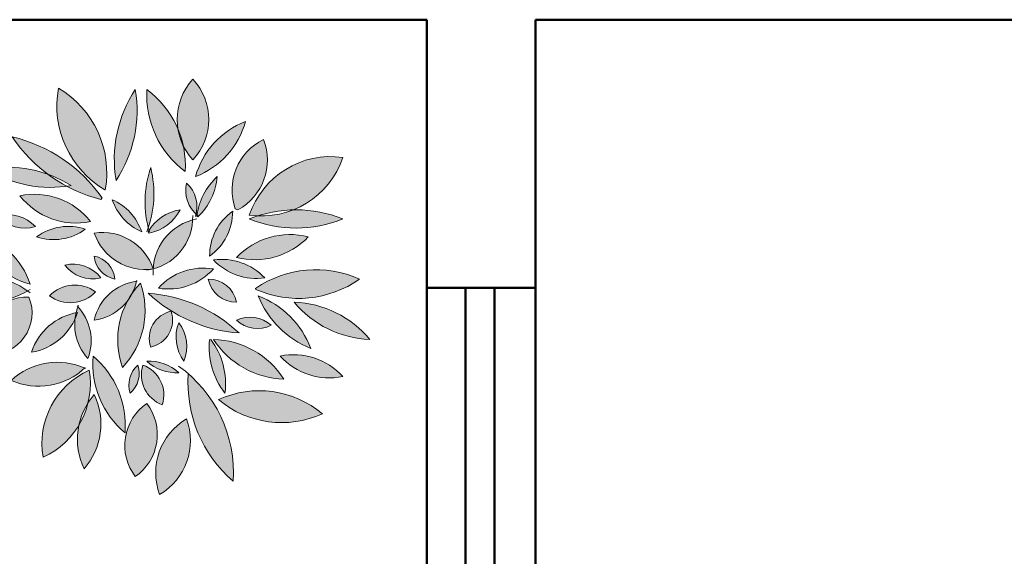
# Model space of a CAD drawing. Units: inches. Extents: x 64 to 1167, y 117 to 939.
# Tile 25 of 56: x 358 to 394, y 837 to 857. Entities that reach past the tile are written whole.
import ezdxf

# ---------------------------------------------------------------- set-up
doc = ezdxf.new("R2010")
doc.units = ezdxf.units.IN
doc.header["$MEASUREMENT"] = 0
doc.layers.add('A-FURN', color=8, linetype='Continuous', lineweight=18)
doc.layers.add('A-WALL', color=7, linetype='Continuous', lineweight=50)

# ---------------------------------------------------------------- blocks, each defined once
blk = doc.blocks.new('A$C172C5132')
at = {"linetype": 'ByBlock'}
h = blk.add_hatch(color=256, dxfattribs=at)
h.set_gradient(color1=(15, 138, 17), color2=(46, 92, 10), tint=1, name='HEMISPHERICAL')
h.paths.add_polyline_path([(0.0848516368565885, 0.0409433570912889, 0.2362815525011606), (0.1000330567823523, 0.0044683605559084, 0.2362815525011239)])
h.paths.add_polyline_path([(0.0951251289552244, 0.0321643424477881, 0.2906279390332829), (0.1303084046611637, 0.0273831593592676, 0.290627939033283)])
h.paths.add_polyline_path([(0.0751445134197123, 6.9582163e-09, 0.3640818940120694), (0.0842661026749416, 0.0256445447606496, 0.3640818940120696)])
h.paths.add_polyline_path([(0.0708009012055837, 0.0308603718690661, 0.4289359753156656), (0.0668916470544005, 0.0060851551611861, 0.4289359753156655)])
h.paths.add_polyline_path([(0.0525577128238133, 0.046942555388035, 0.2430552989308659), (0.0634167555244858, 0.0208633514542425, 0.2430552989308659)])
h.paths.add_polyline_path([(0.0508922599916389, 0.0310927787270394, -0.075691505353723), (0.0477797489950209, 0.0234712737617285, 0.1646663790635834), (0.0495171986775909, 0.0086930668678311, 0.2986360287318925), (0.0529920876610994, 0.0339029598950939, 0.0378503895202349)])
h.paths.add_polyline_path([(0.0356176258998936, 0.0126049410038033, 0.1525669483622997), (0.0477797489950209, 0.0234712737618002, -0.0894079227445343), (0.0508922599916389, 0.0310927787270394, 0.1023004185508453), (0.0512546390377685, 0.0421613668636365, 0.3412881037578929)])
h.paths.add_polyline_path([(0.0247586152468425, 0.0386841445389578, 0.2992020634273156), (0.0497584931614385, 0.0428499944584606, 0.2992020634272661)])
h.paths.add_polyline_path([(0.047451336783066, 0.0636633223899126, 0.031181829370212), (0.0468224604404838, 0.0616275993652971, -0.0067074306643478), (0.047345392022932, 0.0617207568240691), (0.0473453770955458, 0.0617207543709398), (0.0473453802906652, 0.0617207643046988, -0.0313798428369172), (0.0464385188093715, 0.0594096693237134, 0.214704016687058), (0.0508202830851731, 0.0460732317601093, 0.2827951388784949)])
h.paths.add_polyline_path([(0.0643270393991799, 0.0657681421224303, 0.2116588201392034), (0.0625480317599852, 0.0430306771320518, 0.2810507069368319), (0.0686290949419001, 0.0717177787730742, 0.0387724880797508), (0.0658907288251662, 0.0683269518706705, -0.0447168196076769)])
h.paths.add_polyline_path([(0.0529920908817849, 0.0591128495135777, 0.2037329938010539), (0.0643270393991799, 0.0657681421224303, -0.0266555720820853), (0.0658907288251304, 0.0683269518706347, 0.0628291983769196), (0.0672680139649763, 0.0723002515858513, 0.3185820290807026)])
h.paths.add_polyline_path([(0.0694978092295733, 0.0438999815920186, 0.4032574184254003), (0.0760132376538916, 0.0304257186990447, 0.4032574184254003)])
h.paths.add_polyline_path([(0.0651542049250408, 0.0343376032784868, 0.3026067215504981), (0.0677603739667911, 0.0438999851589565, 0.3026067215504981)])
h.paths.add_polyline_path([(0.0708009089365751, 0.0452039393599706, 0.2041900440368323), (0.0816599225525022, 0.0412920661897099, 0.2041900440368324)])
h.paths.add_polyline_path([(0.081659931129825, 0.0582435357128855, 0.2621375963259251), (0.0833973804279365, 0.0452039328038387, 0.2621375963259252)])
h.paths.add_polyline_path([(0.0721039783237091, 0.0499851199959349, 0.4463603731284183), (0.0790537760999147, 0.0621554185296266, 0.4463603731284183)])
h.paths.add_polyline_path([(0.0933876910232543, 0.0525930422323801, 0.2470851436575526), (0.117277559364148, 0.0391187980764294, 0.2470851436575526)])
h.paths.add_polyline_path([(0.0712352546233386, 0.068240566365182, 0.1714668564556485), (0.1020749306824684, 0.054766306652217, 0.1714668564556485)])
h.paths.add_polyline_path([(0.0747101479397659, 0.0699791674706583, 0.2592783200943487), (0.0933876928733241, 0.0764989740396572, 0.2592783200943487)])
h.paths.add_polyline_path([(0.0916502366687461, 0.0730217515827079, 0.3656390256905797), (0.101206201234342, 0.0651979848924216, 0.3656390256905797)])
h.paths.add_polyline_path([(0.0933876912086265, 0.0795415399056317, 0.2434153457947699), (0.1107621376206411, 0.0734563950534696, 0.2434153457947698)])
h.paths.add_polyline_path([(0.1012061854802825, 0.0591128377539187, 0.3074508191165638), (0.1129339572098902, 0.0573742297376074, 0.3074508191165636)])
h.paths.add_polyline_path([(0.1085903436375709, 0.0673712529429685, 0.2096325949128592), (0.1263991528693673, 0.0495504795221731, 0.2096325949128592)])
h.paths.add_polyline_path([(0.1207524492141115, 0.065197986908134, 0.2131103218534129), (0.1463797799587205, 0.0525930392730849, 0.2131103218534128)])
h.paths.add_polyline_path([(0.1159744952746058, 0.0469425441179992, 0.2657190469918038), (0.1372581767641242, 0.039988102251266, 0.2657190469918037)])
h.paths.add_polyline_path([(0.1012062017913538, 0.0804108456417557, 0.2715342573869963), (0.1255304209675389, 0.0873652998785119, 0.2715342573869963)])
h.paths.add_polyline_path([(0.1203979563089573, 0.0965262847971841, -0.1054095226912168), (0.1084157654269272, 0.0944920995295244, 0.018051737402885), (0.1055497991297656, 0.0934504485621891, 0.1947634324622436), (0.1372581839236379, 0.0934504485621891, 0.1024884098922396)])
h.paths.add_polyline_path([(0.1055498097535589, 0.0947544097676372, 0.0247013481528025), (0.1084157654269988, 0.0944920995295244, -0.0722993566674296), (0.1203979563089573, 0.0965262847971841, 0.2204439691458661), (0.1372581853767884, 0.1143137971598573, 0.3612839562176665)])
h.paths.add_polyline_path([(0.0920846062711383, 0.0808455117020383, 0.2441882660981068), (0.0999031055369228, 0.0960583567237383, 0.2441882660981067)])
h.paths.add_polyline_path([(0.0873066344977665, 0.1077940073224099, 0.2360393724983017), (0.104246714262817, 0.1264840796844728, 0.2360393724983016)])
h.paths.add_polyline_path([(0.0842661033232609, 0.1056207182491079, 0.2718871002718489), (0.0875115893454784, 0.0950658132315734, 0.2718871002715955)])
h.paths.add_polyline_path([(0.0729522379931478, 0.076559000959958, -0.0011928136807371), (0.072980246539008, 0.0764766754647066, 0.3253441804237751), (0.0863528333196324, 0.0931339331977748, 0.3244683045754948)])
h.paths.add_polyline_path([(0.0712894635586684, 0.0904598878984896, 0.1439511720342415), (0.0721039819483319, 0.1108365706518253, 0.1439511720343805)])
h.paths.add_polyline_path([(0.0590731413665092, 0.0999702409597207, 0.2079760795555611), (0.0690634560800835, 0.0891039085706064, 0.207976079555561)])
h.paths.add_polyline_path([(0.0603762293124555, 0.1064900535994177, 0.1901074032574417), (0.0668916420391818, 0.137350397132487, 0.1901074032574415)])
h.paths.add_polyline_path([(0.0708008986345782, 0.1373504136971785, 0.2529037224987196), (0.0838317360148722, 0.1095326193878703, 0.0679209033287059), (0.083148370263475, 0.1182431328493921, -0.0747956075290694), (0.0813338508249389, 0.1239670055877479, 0.1341585858806744)])
h.paths.add_polyline_path([(0.0813338508249389, 0.1239670055877479, -0.0465642878043537), (0.083148370263475, 0.1182431328493921, 0.0724450463034802), (0.086437905090639, 0.1134444986822172, 0.3910737637767219), (0.086437905090639, 0.140827633644925, 0.2297305268739758)])
h = blk.add_hatch(color=256, dxfattribs=at)
h.set_gradient(color1=(12, 110, 14), color2=(39, 78, 9), tint=1, name='HEMISPHERICAL')
h.paths.add_polyline_path([(0.0277991349999923, 0.1012741996741918, 0.2872652564561664), (0.0516889943617385, 0.0925811437956438, 0.2872652564561664)])
h.paths.add_polyline_path([(0.0334458088073508, 0.0873652986886136, 0.2454535408657207), (0.0499515759045565, 0.089973222633763, 0.2454535408657209)])
h.paths.add_polyline_path([(0.0529920764399042, 0.0886692609657258, 0.3628842943462125), (0.0729490150136937, 0.0764954078429701, -0.0008769890010568), (0.0729522379931478, 0.076559000959958, 0.362271709300998)])
h.paths.add_polyline_path([(0.052992082253688, 0.0808454969822246, 0.3332704001676869), (0.0599418568393184, 0.0730217437701484, 0.3332704001676869)])
h.paths.add_polyline_path([(0.0430017763078933, 0.0778029274210876, 0.3029447989434044), (0.055163891633107, 0.0734563959517209, 0.3029447989434045)])
h.paths.add_polyline_path([(0.0377894338124123, 0.0673712519411278, 0.378762981535274), (0.0534264495230472, 0.0686752079740218, 0.378762981535274)])
h.paths.add_polyline_path([(0.0317083892186356, 0.0482465196716572, 0.2476978196244638), (0.0464385188093715, 0.059409669323785, -0.03294569524484), (0.046822460440448, 0.0616275993652971, 0.2740394890495783)])
h.paths.add_polyline_path([(0.0169400999274739, 0.0473772010126878, 0.5498076116501301), (0.0308396477386464, 0.0669366019959097, 0.5498076116501304)])
h.paths.add_polyline_path([(5.8794536e-09, 0.0704138252261443, 0.2977812259051555), (0.030406089434854, 0.069011140085252, 0.2977812259051677)])
h.paths.add_polyline_path([(0.0130308377588801, 0.0886692600222146, 0.2481107794618412), (0.0312740176044698, 0.0712831333595387, 0.2481107794618409)])
h.paths.add_polyline_path([(0.0204149782987906, 0.0943197520353183, 0.2904151352643436), (0.0330114769075243, 0.09084252142568, 0.2904151352643436)])
h.paths.add_polyline_path([(0.0165057375983538, 0.1104019119840517, 0.1754058278069592), (0.0436644963260339, 0.1045192247680393, -0.0373225713202712), (0.0372078839723324, 0.1086182328550855, 0.1293741954878769)])
h.paths.add_polyline_path([(0.0251929565725431, 0.1212682457447485, 0.0856466426118782), (0.0372078839723682, 0.1086182328550855, -0.0543838481538954), (0.04517356720194, 0.1047514234187564), (0.0451735772956124, 0.1047514251656665, -0.009350805838724), (0.0436644963260339, 0.1045192247680393, 0.0605073730854804), (0.0551972396525293, 0.1000437593582652), (0.0556053915159454, 0.1006328511779318, 0.1852537253176007)])
h.paths.add_polyline_path([(0.0408299697457594, 0.137785076184794, 0.3132662906545535), (0.0565859837452511, 0.103262326620679), (0.0567280634683676, 0.1033275296575847, 0.313266248548697)])
h.paths.add_polyline_path([(0.0712352633028543, 0.0891039098711838), (0.0715593597632914, 0.0886487531724155, 0.2302319040247018), (0.0820942930736631, 0.0964930128417399, 0.2302320083900739)])
h.paths.add_polyline_path([(0.0877409962472449, 0.094319752764776), (0.0881219586038091, 0.0941299738834785, 0.1793447999456611), (0.0946907683226341, 0.1077939919612951, 0.179344717845649)])
h.paths.add_polyline_path([(0.1007774209509037, 0.0968245554685736), (0.1016405548364666, 0.0964930185287673, 0.3782823007975571), (0.110327781776827, 0.120398949988467, 0.3782823000244757)])
h = blk.add_hatch(color=256, dxfattribs=at)
h.set_gradient(color1=(12, 110, 14), color2=(39, 78, 9), tint=1, name='HEMISPHERICAL')
h.paths.add_polyline_path([(0.1076878936631927, 0.0699044517198683), (0.1077216139834834, 0.0695445217982392, 0.2622438465353351), (0.1429048742833344, 0.0730217411596838, 0.2622438895928425)])
h = blk.add_hatch(color=256)
h.set_gradient(color1=(12, 110, 14), color2=(39, 78, 9), tint=1, name='HEMISPHERICAL')
h.paths.add_polyline_path([(0.0925189745611727, 0.0525930461325369), (0.0920047978464449, 0.0524506733356022, 0.1924721118722921), (0.0972969476804535, 0.034337589023518, 0.1924721317293766)])
for p, q in [((0.0551972396525293, 0.1000437593582652), (0.0556053915159454, 0.1006328511779318)), ((0.0565859837452511, 0.103262326620679), (0.0567280634683676, 0.1033275296575847)), ((0.1016405548364666, 0.0964930185287673), (0.1007774209509037, 0.0968245554685736)), ((0.0881219586038091, 0.0941299738834785), (0.0877409962472449, 0.094319752764776)), ((0.0715593597632914, 0.0886487531724155), (0.0712352633028543, 0.0891039098711838)), ((0.1077216139834834, 0.0695445217982392), (0.1076878936631927, 0.0699044517198683)), ((0.0925189745611727, 0.0525930461325369), (0.0920047978464449, 0.0524506733356022))]:
    blk.add_line(p, q, dxfattribs=at)
for centre, radius, start, end in [((0.101265794581761, 0.1271360661635711), 0.0201823023180461, 137.2816499999981, 222.7183500000019), ((0.0716100155995529, 0.1271360661635711), 0.0201823023180461, 317.2816499999981, 42.71835000000189), ((0.0735549152138597, 0.1318637225567745), 0.0332563450288768, 169.7436950000113, 239.3197540000017), ((0.0239790024348321, 0.1091140213495727), 0.0332563450288768, 349.979727, 59.55578500000095), ((0.10275001526468, 0.1136618142921691), 0.0429764108245464, 146.5506230000061, 189.606293999996), ((0.0245178560869572, 0.130178636439664), 0.0429764108245464, 326.5506230000061, 9.606293999996069), ((0.1030559147706098, 0.1354988531099791), 0.0323081157380791, 176.7145950000032, 233.4855010000019), ((0.0515767198788405, 0.1113841799750697), 0.0323081157380791, 356.7145950000031, 53.48550100000192), ((0.0770840696856873, 0.1340814184931329), 0.0282051204109551, 291.2498849999908, 344.3738200000102), ((0.1144692790748961, 0.1001966685137141), 0.0282051204109551, 111.2498849999908, 164.3738200000101), ((0.0135073941244871, 0.0713174556861172), 0.0512994522116023, 34.85184100001269, 76.83293799999853), ((0.0678545735110574, 0.1497571951357996), 0.0512994522116023, 213.7345550000018, 255.7156519999993), ((0.1189030526233196, 0.1032032733459664), 0.0192152690661484, 116.5048729999953, 199.3878370000049), ((0.0924459638948487, 0.1133656609626513), 0.0192152690661484, 298.5877680000021, 21.47073299999085), ((0.1331720103728117, 0.0854565851877726), 0.0291450769250325, 81.94051299999644, 161.396420999996), ((0.1096359847575714, 0.1236116217397935), 0.0291450769250325, 261.9405129999964, 341.396420999996), ((0.0234677569105627, 0.0701752569545988), 0.0408246676381128, 57.88070199999403, 99.81891900000039), ((0.0382115478896952, 0.1449780784482092), 0.0408246676381128, 237.880701999994, 279.8189190000004), ((0.1063515957832179, 0.0992629679096916), 0.0361503434813414, 161.3278780000036, 196.3784880000011), ((0.0370418497237108, 0.1020334906406949), 0.0361503434813414, 339.0433640000005, 14.0939750000002), ((0.1093943472150794, 0.0916807446201365), 0.0218135731168313, 132.3808890000008, 173.0513299999991), ((0.0729718716492938, 0.1098241395953668), 0.0218135731168313, 313.9894330000009, 354.6598739999948), ((0.0948766385427795, 0.1031068864394069), 0.0109042564172143, 166.6712360000006, 231.5787619999986), ((0.0769010541259599, 0.0975796450412743), 0.0109042564172143, 342.6050669999977, 47.51259299999652), ((0.0466851175819402, 0.1160027564860523), 0.0239501716871959, 217.949471999991, 282.0595879999972), ((0.0328030117797547, 0.0778525869838191), 0.0239501716871959, 37.94947199999101, 102.0595879999972), ((0.0765653122385901, 0.1060266090005227), 0.0185109598796141, 199.0975429999934, 246.0922180000009), ((0.0515712852079667, 0.0830475405298402), 0.0185109598796141, 19.09754299999351, 66.09221800000086), ((0.0294540951469793, 0.1025101112732027), 0.0121978530012546, 222.1798159999954, 286.9561240000028), ((0.0239723600593714, 0.0826521621877956), 0.0121978530012546, 42.17981599999539, 106.9561240000027), ((0.0682216553335405, 0.0939933540633402), 0.0181515349044702, 278.3255549999997, 1.781575000010764), ((0.0842630162449453, 0.081632086548538), 0.0150183384728482, 98.30281699999492, 150.1643819999994), ((0.0687605452167835, 0.1034039938555789), 0.0150183384728482, 280.7404219999926, 332.601987000013), ((0.1106400703875398, 0.0809246494070092), 0.0185556328739039, 125.3546809999916, 180.2443949999947), ((0.0813476414204855, 0.0959792190187316), 0.0185556328739039, 305.3546809999916, 0.2443949999947113), ((0.121403991526648, 0.0542932043610051), 0.0422450611313307, 67.95770299999826, 112.0422970000017), ((0.0441948910186934, 0.0728706121494062), 0.0180454622067554, 71.39698899999804, 126.5601259999975), ((0.0910788664069822, 0.0756084423160586), 0.0181515349044702, 100.5963680000002, 184.0523880000084), ((0.121403991526648, 0.1326076927634088), 0.0422450611313307, 247.9577029999983, 292.0422970000018), ((0.0385925183154827, 0.0972267054400285), 0.0269560639736953, 198.5093169999973, 254.2466049999954), ((0.0057123370479029, 0.0627256879417248), 0.0269560639736953, 18.50931699999731, 74.24660499999541), ((0.0392024936932855, 0.1044679091729345), 0.0180454622067554, 251.396988999998, 306.5601259999975), ((0.070252990368267, 0.094520649982155), 0.018225748354027, 198.7264799999882, 278.5819429999999), ((0.0557117918409013, 0.0706475781585839), 0.018225748354027, 18.72647999998828, 98.58194299999985), ((0.1074374792478634, 0.1046320241552055), 0.0250098841924539, 255.5725970000049, 316.3385330000025), ((0.1192991435110293, 0.063144121365062), 0.0250098841924539, 75.57259700000495, 136.3385330000025), ((0.0512499029286849, 0.0722993437049655), 0.008721922072485, 4.75100299999709, 78.4778570000038), ((0.0616840361643215, 0.0815678970473717), 0.008721922072485, 184.751002999997, 258.4778570000038), ((0.0458251231914507, 0.0665141969829806), 0.0116364394266253, 36.62615099999231, 104.0418149999998), ((0.0523405447495496, 0.0847451263898996), 0.0116364394266253, 216.6261509999923, 284.0418149999998), ((0.0899128034319171, 0.056440575656638), 0.0203571658715258, 80.1716990000048, 138.3135889999978), ((0.0961954640765332, 0.0597118248046133), 0.0200275108155287, 43.33670399999354, 98.05919799999388), ((0.1079543647527345, 0.0932861101545596), 0.0200275108155287, 223.3367039999936, 278.0591979999939), ((0.0141298571681875, 0.0464488729354848), 0.0278203457156127, 52.09546799999781, 120.5238170000041), ((0.0781850373811729, 0.0900375658536775), 0.0203571658715258, 260.1716990000048, 318.3135889999978), ((0.1280637579422302, 0.0401992188583729), 0.0360218920168197, 65.66928900000572, 124.4475970000009), ((0.0162762381460842, 0.0929760923759115), 0.0278203457156127, 234.1936160000109, 302.6219659999903), ((0.0463451366513398, 0.0591828018681872), 0.0118427516086885, 53.27718599999966, 136.2564700000069), ((0.0508318559707725, 0.0757722432951048), 0.0167988694869422, 277.3883189999978, 349.0702710000075), ((0.0694282488759529, 0.0556408578043242), 0.0167988694869422, 96.39019900000564, 168.0721500000032), ((0.0890906585045813, 0.0523922772722525), 0.028145169953087, 136.6355579999986, 199.4277959999973), ((0.0420864681973041, 0.0623561786328734), 0.028145169953087, 316.6355579999986, 19.42779599999733), ((0.1010624291989654, 0.0747701020695983), 0.0095731968355297, 190.5230030000053, 270.8604580000047), ((0.0917940087040512, 0.0634496344054954), 0.0095731968355297, 10.52300300000533, 90.86045800000468), ((0.1222263417638192, 0.1025170797289037), 0.0360218920168197, 246.2551610000005, 305.0334690000088), ((0.030095144764983, 0.0527472337402677), 0.0142088865211648, 86.99645899999618, 202.2057780000005), ((0.0176846029012089, 0.061566569268294), 0.0142088865211648, 266.9964589999962, 22.20577800000054), ((0.0448707466840482, 0.0768636580469624), 0.0118427516086885, 233.2771859999997, 316.2564700000069), ((0.0675871152435055, 0.0178609463876896), 0.0505115336334844, 46.93944700000039, 85.85825999999756), ((0.1057230700623015, 0.1051459266297094), 0.0505115336334844, 226.9394470000004, 265.8582599999975), ((0.1378131830374621, 0.0787656599927382), 0.0313656955065552, 201.3015170000018, 248.6599970000021), ((0.0971763134694045, 0.0381560724723318), 0.0313656955065552, 21.30151700000185, 68.65999700000215), ((0.0634424178754735, 0.0576083535722988), 0.0170990444729038, 157.7122499999933, 222.4235080000054), ((0.0348292019927655, 0.0521282005777588), 0.0170990444729038, 339.2610190000014, 43.97227699999542), ((0.1476814341913268, 0.0875936064547896), 0.0350247627655248, 219.748773000006, 267.8701689999957), ((0.1194507949815051, 0.0301974197264293), 0.0350247627655248, 39.74877300000596, 87.87016899999576), ((0.0284978225433556, 0.0677829752368411), 0.0197985058634545, 279.3323689999943, 342.1699049999944), ((0.0505559437708258, 0.0421842988057918), 0.0197985058634545, 99.33236899999434, 162.1699049999945), ((0.081037200945223, 0.0529533164584823), 0.0094134295899337, 102.1635449999909, 198.3798429999994), ((0.0701205534784725, 0.0591872220671508), 0.0094134295899337, 282.1635449999909, 18.37984299999946), ((0.1057899768988151, 0.0496086630230044), 0.0105517998977895, 47.38731500000322, 115.7475850000102), ((0.0941099514120365, 0.0532668728117116), 0.0134078401937111, 158.2118580000032, 216.9673489999941), ((0.0709473601456892, 0.0501805957050126), 0.0134078401937111, 338.2118580000033, 36.96734899999409), ((0.1083501657913576, 0.0668784044684502), 0.0105517998977895, 227.3873150000032, 295.7475850000102), ((0.1173062014065116, 0.0500134010759287), 0.0254185231312991, 174.4977019999966, 218.0761069999966), ((0.0720745591857262, 0.0374891658982219), 0.0254185231312991, 352.877761000004, 36.45616599999835), ((0.1181335032326502, 0.0685519086981837), 0.0294455538371517, 212.8184350000037, 268.3342569999997), ((0.0925317471547521, 0.0231599316106257), 0.0294455538371517, 32.8184350000037, 88.33425699999965), ((0.0832269143652089, 0.044412429310089), 0.0307733888474724, 175.2839350000003, 229.928474000003), ((0.0327475539830902, 0.0233934775321169), 0.0307733888474724, 355.2839350000003, 49.92847400000303), ((0.1205352775087439, 0.0248545827484154), 0.0225539081324995, 42.14373300000566, 101.6666580000013), ((0.1326973945299862, 0.0620760636208497), 0.0225539081324995, 222.1437330000056, 281.6666580000013), ((0.0404277462722728, 0.0217482818989244), 0.0230726051943408, 65.4893189999949, 132.7751640000022), ((0.0736338870196566, 0.0371628561840394), 0.0089379562768254, 131.0823399999971, 198.426954999994), ((0.0592806918721395, 0.0410747322533682), 0.0089379562768254, 311.0823399999972, 18.42695499999411), ((0.079750512431678, 0.040545250389174), 0.0107875921498883, 161.8816990000004, 249.730113000004), ((0.0657605344518227, 0.0337804499018535), 0.0107875921498883, 341.8816990000004, 69.73011300000398), ((0.0716406067578116, 0.0305070993478934), 0.0147208083600278, 47.10765200001037, 93.27005900000032), ((0.0808202247312299, 0.055988906201823), 0.0147208083600278, 227.1076520000103, 273.2700590000003), ((0.0560042133631615, 0.0075397818432334), 0.0441358435011617, 356.0095630000061, 54.57675200000271), ((0.0340893621360082, 0.059785857098494), 0.0230726051943408, 246.1459300000069, 313.4317750000005), ((0.0625649600760164, 0.0172629272857448), 0.0273469496544691, 114.430325999999, 189.8069550000016), ((0.0243073048616458, 0.0375033805817666), 0.0273469496544691, 294.430325999999, 9.806955000001677), ((0.1288804802757793, 0.0378719358038923), 0.0441358435011617, 176.0095630000062, 229.1860109999974), ((0.0704766934969721, 0.0186484785003509), 0.0232036773779111, 138.8968619999938, 205.406926999994), ((0.0320325928417182, 0.0239475482625383), 0.0232036773779111, 318.8968619999938, 25.40692699999402), ((0.1089513490794741, 0.0020651842900081), 0.033122857436045, 49.85059000000689, 114.6719470000004), ((0.0806294557077931, 0.0166135082746334), 0.0173081947608492, 124.6008150000011, 217.4657849999944), ((0.0570630925521911, 0.0203320187555472), 0.0173081947608492, 304.6008150000012, 37.4657849999944), ((0.1164821845369855, 0.0574823175170118), 0.033122857436045, 229.8505900000069, 294.6719470000005), ((0.0949801750607728, 0.0073891086135142), 0.0211672458296172, 120.4085659999984, 200.4311790000044), ((0.0644304410338453, 0.0182554431053159), 0.0211672458296172, 300.4085659999984, 20.43117900000441)]:
    blk.add_arc(centre, radius, start, end, dxfattribs=at)

msp = doc.modelspace()

# ---------------------------------------------------------------- linework, layer by layer
at = {"layer": 'A-WALL'}
for p, q in [((373.1072888543382, 857.1997537567943), (301.1072888543381, 857.1997537567943)), ((373.1072888543381, 857.1997537567943), (373.1072888543381, 847.3108866272732)), ((467.107288854338, 857.1997537567943), (377.1072888543382, 857.1997537567943)), ((377.107288854338, 857.1997537567943), (377.1072888543382, 823.3108866272732)), ((373.1072888543381, 847.3108866272732), (373.107288854338, 785.1997537567942)), ((373.1072888543381, 847.3108866272732), (377.1072888543381, 847.3108866272732)), ((374.5240759622134, 847.3108866272732), (374.5240759622134, 823.3108866272731)), ((375.5949572653144, 847.3108866272732), (375.5949572653144, 823.3108866272731)), ((377.1072888543381, 847.3108866272732), (377.107288854338, 785.1997537567942))]:
    msp.add_line(p, q, dxfattribs=at)

# ---------------------------------------------------------------- block references
at = {"layer": 'A-FURN', "xscale": 108.7946212322529, "yscale": 108.7946212322529, "zscale": 108.7946212322529}
msp.add_blockref('A$C172C5132', (355.0733037585648, 839.6808550028877), dxfattribs=at)

doc.saveas('drawing.dxf')
